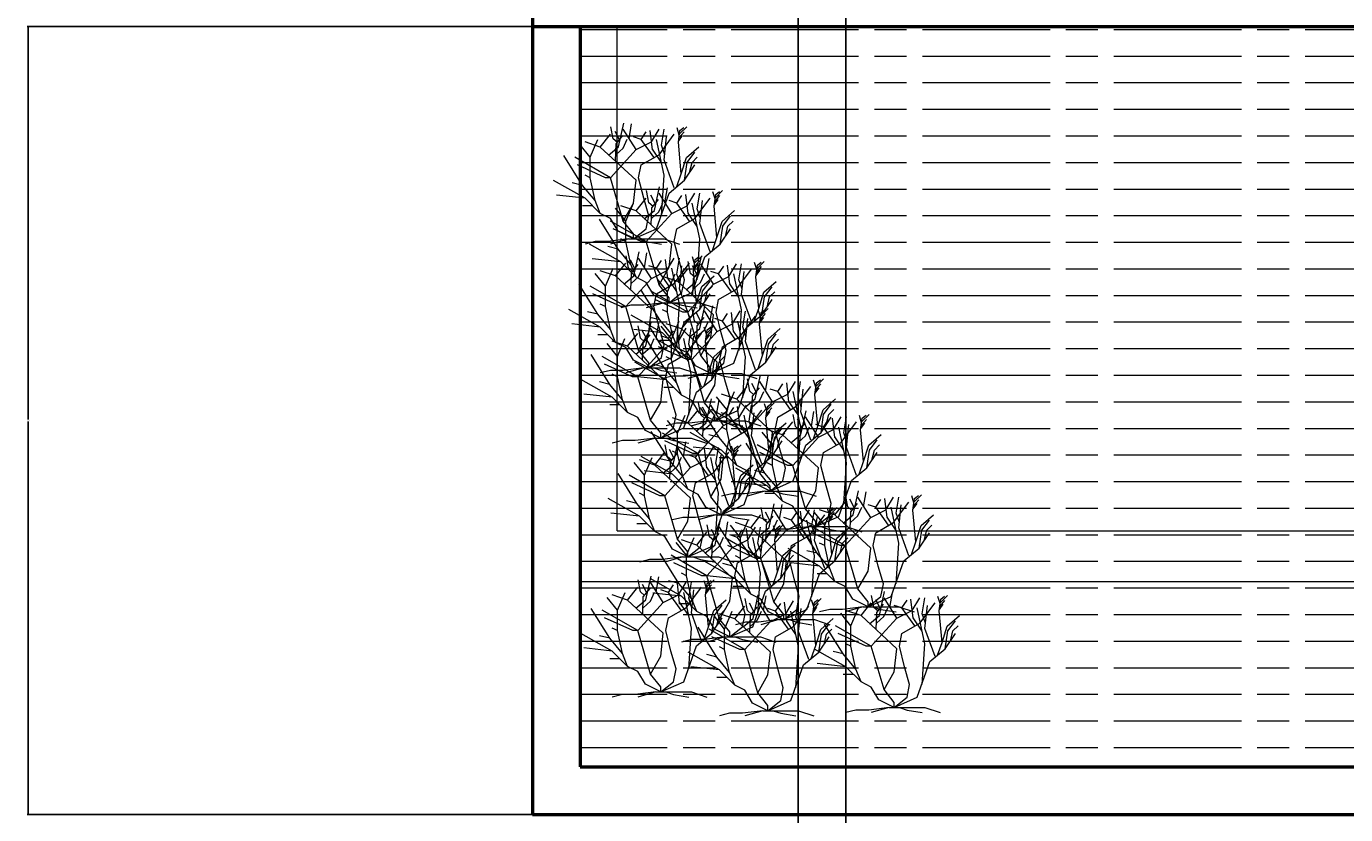
# Model space of a CAD drawing. Units: inches. Extents: x 5375 to 6084, y 16106 to 17259.
# Tile 2 of 32: x 5375 to 5624, y 16212 to 16361. Entities that reach past the tile are written whole.
import ezdxf

# ---------------------------------------------------------------- set-up
doc = ezdxf.new("R2010")
doc.units = ezdxf.units.IN
for name, color, linetype, lineweight in [('A-ANNO-DIMS', 2, 'Continuous', 18), ('C-PVMT-PATT', 2, 'Continuous', 13), ('L-PLNT-TREE', 3, 'Continuous', 13), ('WALL', 6, 'Continuous', 50)]:
    doc.layers.add(name, color=color, linetype=linetype, lineweight=lineweight)
doc.styles.get("Standard").update_dxf_attribs({"font": 'arial.ttf'})
doc.dimstyles.get("Standard").update_dxf_attribs({"dimtxt": 0.18, "dimasz": 0.18, "dimexe": 0.18, "dimexo": 0.0625, "dimgap": 0.09, "dimtad": 0, "dimtih": 1, "dimtoh": 1, "dimdec": 4, "dimzin": 0, "dimdsep": 46, "dimtxsty": 'Standard', "dimcen": 0.09, "dimadec": 0, "dimazin": 0, "dimtfac": 1, "dimtdec": 4, "dimtofl": 0, "dimtmove": 0, "dimatfit": 3, "dimfxl": 1, "dimtolj": 1, "dimtzin": 0, "dimarcsym": 0})

# ---------------------------------------------------------------- blocks, each defined once
blk = doc.blocks.new('*U12')
for p, q in [((-11.433, 18.289), (-10.457, 22.749)), ((-9.48, 19.775), (-8.992, 22.592)), ((-14.88, 18.24), (-12.96, 20.64)), ((-12.471, 19.775), (-12.898, 22.044)), ((-11.28, 19.619), (-12.104, 21.184)), ((-11.921, 18.836), (-10.64, 20.401)), ((-8.16, 17.76), (-10.56, 21.6)), ((-7.2, 19.68), (-8.64, 20.16)), ((-7.2, 19.68), (-6.24, 21.12)), ((-5.086, 17.741), (-5.513, 21.34)), ((-5.28, 19.2), (-3.84, 21.6)), ((-3.84, 16.8), (-0.96, 20.64)), ((-3.377, 18.602), (-2.888, 21.575)), ((-2.88, 15.84), (-2.4, 20.16)), ((-0.508, 21.888), (-0.081, 20.558)), ((-0.203, 19.149), (0.102, 21.34)), ((-0.142, 19.384), (0.59, 20.401)), ((-0.02, 20.01), (0.896, 21.105)), ((0.041, 20.714), (1.384, 22.044)), ((0.102, 21.34), (0.835, 21.888)), ((-16.8, 16.32), (-18.72, 18.72)), ((-14.88, 18.24), (-17.76, 19.2)), ((-16.8, 16.32), (-15.36, 19.68)), ((-8.16, 12), (-14.88, 18.24)), ((-13.325, 16.724), (-11.433, 18.289)), ((-12.96, 12.48), (-8.16, 17.76)), ((-11.677, 19.071), (-12.471, 19.775)), ((-12.043, 15.628), (-11.921, 18.836)), ((-11.982, 16.802), (-10.579, 18.054)), ((-10.579, 18.054), (-9.846, 19.697)), ((-8.16, 17.76), (-5.28, 19.2)), ((-4.8, 16.32), (-7.2, 19.68)), ((-3.377, 15.315), (-5.086, 17.819)), ((-2.88, 12.96), (-4.32, 19.68)), ((-2.766, 16.802), (-3.377, 18.602)), ((0.346, 13.203), (-0.203, 19.149)), ((1.323, 16.254), (3.642, 18.289)), ((-18.24, 11.04), (-21.755, 16.655)), ((-12.96, 12.48), (-19.68, 16.32)), ((-16.8, 12.48), (-16.8, 16.32)), ((-7.2, 14.88), (-3.84, 16.8)), ((-0.96, 10.56), (-2.88, 15.84)), ((0.346, 13.203), (1.323, 16.254)), ((0.96, 12), (1.44, 15.36)), ((1.44, 15.36), (2.88, 17.28)), ((1.92, 13.44), (2.4, 15.36)), ((2.4, 15.36), (3.36, 16.32)), ((-13.92, 12.48), (-19.2, 14.88)), ((-16.8, 12.48), (-17.76, 12.96)), ((-15.84, 8.16), (-16.8, 12.48)), ((-12.96, 12.48), (-13.92, 12.48)), ((-10.56, 4.32), (-12.96, 12.48)), ((-7.68, 12.48), (-7.2, 14.88)), ((-6.72, 8.64), (-7.68, 12.48)), ((-3.36, 5.28), (-2.88, 12.96)), ((-0.48, 10.8), (0.346, 13.203)), ((0.96, 12), (2.88, 14.88)), ((-17.76, 8.64), (-23.663, 11.961)), ((-18.24, 11.04), (-20.16, 11.52)), ((-15.84, 8.16), (-18.24, 11.04)), ((-8.64, 7.68), (-8.16, 12)), ((-1.92, 9.6), (0.96, 12)), ((-17.76, 8.64), (-23.128, 9.222)), ((-14.88, 5.76), (-17.76, 8.64)), ((-14.88, 5.76), (-15.84, 8.16)), ((-10.56, 4.32), (-8.64, 7.68)), ((-5.76, 5.28), (-6.72, 8.64)), ((-4.32, 2.88), (-1.92, 9.6)), ((-16.32, 7.2), (-18.24, 7.2)), ((-12.96, 4.8), (-14.88, 5.76)), ((-6.24, 2.88), (-5.76, 5.28)), ((-11.52, 2.4), (-12.96, 4.8)), ((-8.64, 1.92), (-10.56, 4.32)), ((-8.64, 0.96), (-4.32, 2.88)), ((-8.64, 0.96), (-6.24, 2.88)), ((-15.84, 0.48), (-17.76, 0)), ((-13.44, 0.48), (-15.84, 0.48)), ((-9.6, 0.96), (-13.44, 0.48)), ((-9.6, 0.96), (-12.96, 0)), ((-8.64, 0.96), (-11.52, 2.4)), ((-9.6, 0.96), (-7.68, 0.96)), ((-8.64, 0.96), (-8.64, 1.92)), ((-8.64, 0.96), (-2.88, 0.96)), ((-7.68, 0.96), (-6.24, 0.48)), ((-6.24, 0.48), (-3.36, 0)), ((-2.88, 0.96), (0, 0))]:
    blk.add_line(p, q)
blk = doc.blocks.new('*D33')
at = {"layer": 'A-ANNO-DIMS', "color": 0, "lineweight": -2, "transparency": 16777216}
for p, q in [((5470.56, 16360.58), (5375.56, 16360.58)), ((5375.74, 16360.4), (5375.74, 16286.66)), ((5375.74, 16212.56), (5375.74, 16286.3)), ((5470.56, 16212.38), (5375.56, 16212.38))]:
    blk.add_line(p, q, dxfattribs=at)
at = {"layer": 'A-ANNO-DIMS', "color": 0, "transparency": 16777216}
for points in [[(5375.71, 16360.4), (5375.77, 16360.4), (5375.74, 16360.58)], [(5375.71, 16212.56), (5375.77, 16212.56), (5375.74, 16212.38)]]:
    blk.add_solid(points, dxfattribs=at)
at = {"layer": 'Defpoints', "color": 0, "transparency": 16777216}
for p in [(5375.74, 16360.58), (5470.62, 16360.58), (5470.62, 16212.38)]:
    blk.add_point(p, dxfattribs=at)
at = {"layer": 'A-ANNO-DIMS', "color": 0, "transparency": 16777216, "insert": (5375.74, 16286.48), "char_height": 0.18, "attachment_point": 5}
blk.add_mtext('\\A1;148.2', dxfattribs=at)
blk = doc.blocks.new('*D40')
at = {"layer": 'A-ANNO-DIMS', "color": 0, "lineweight": -2, "transparency": 16777216}
for p, q in [((5529.62, 16876.52), (5529.62, 16106.48)), ((5520.62, 16867.52), (5520.62, 16106.48)), ((5520.8, 16106.66), (5524.97, 16106.66)), ((5529.44, 16106.66), (5525.27, 16106.66))]:
    blk.add_line(p, q, dxfattribs=at)
at = {"layer": 'A-ANNO-DIMS', "color": 0, "transparency": 16777216}
for points in [[(5520.8, 16106.69), (5520.8, 16106.63), (5520.62, 16106.66)], [(5529.44, 16106.69), (5529.44, 16106.63), (5529.62, 16106.66)]]:
    blk.add_solid(points, dxfattribs=at)
at = {"layer": 'Defpoints', "color": 0, "transparency": 16777216}
for p in [(5529.62, 16876.58), (5520.62, 16867.58), (5529.62, 16106.66)]:
    blk.add_point(p, dxfattribs=at)
at = {"layer": 'A-ANNO-DIMS', "color": 0, "transparency": 16777216, "insert": (5525.12, 16106.66), "char_height": 0.18, "attachment_point": 5}
blk.add_mtext('\\A1;9', dxfattribs=at)

msp = doc.modelspace()

# ---------------------------------------------------------------- hatches: boundary and pattern name
at = {"layer": 'C-PVMT-PATT'}
h = msp.add_hatch(dxfattribs=at)
h.set_pattern_fill('AR-B816C', color=256)
h.paths.add_polyline_path([(5707.6199, 16360.5793), (5479.6199, 16360.5793), (5479.6199, 16221.3785), (5802.2897, 16221.3785, 0.20288708), (5707.6199, 16299.0135)])
h = msp.add_hatch(dxfattribs=at)
h.set_pattern_fill('ACAD_ISO08W100', color=256)
h.paths.add_polyline_path([(5707.6199, 16360.5793), (5479.6199, 16360.5793), (5479.6199, 16221.3785), (5802.2897, 16221.3785, 0.20288708), (5707.6199, 16299.0135)])

# ---------------------------------------------------------------- linework, layer by layer
at = {"layer": 'WALL'}
for p, q in [((5470.6199, 16603.5793), (5470.6199, 16212.3785)), ((5470.6199, 16360.5793), (5707.6199, 16360.5793)), ((5479.6199, 16360.5793), (5479.6199, 16221.3785)), ((5479.6199, 16221.3785), (6022.6199, 16221.3785)), ((5470.6199, 16212.3785), (6031.6199, 16212.3785))]:
    msp.add_line(p, q, dxfattribs=at)

# ---------------------------------------------------------------- block references
at = {"layer": 'L-PLNT-TREE'}
for p in [(5498.2883, 16319.6538), (5505.0083, 16307.6538), (5501.1683, 16295.4138), (5512.8569, 16294.35), (5513.5769, 16285.47), (5503.4089, 16282.212), (5523.9837, 16272.2398), (5514.757, 16267.7776), (5532.5845, 16265.5668), (5508.517, 16259.8576), (5542.4264, 16250.4777), (5526.5864, 16248.0777), (5516.4184, 16244.8197), (5503.4193, 16234.4827), (5523.578, 16230.9501), (5547.3447, 16231.5511)]:
    msp.add_blockref('*U12', p, dxfattribs=at)

# ---------------------------------------------------------------- dimensions: what is measured, and where the dimension line sits
at = {"layer": 'A-ANNO-DIMS'}
dim = msp.add_linear_dim(base=(5529.6199, 16106.6631), p1=(5520.6199, 16867.5793), p2=(5529.6199, 16876.5793), dimstyle='Standard', override={"dimdec": 0, "dimlfac": 1, "dimrnd": 0, "dimzin": 0, "dimdsep": 46, "dimlunit": 2}, dxfattribs=at)
dim.commit()
dim.dimension.update_dxf_attribs({"geometry": '*D40', "text_midpoint": (5525.1199, 16106.6631)})
dim = msp.add_linear_dim(base=(5375.7423, 16360.5793), p1=(5470.6199, 16212.3785), p2=(5470.6199, 16360.5793), angle=90, dimstyle='Standard', override={"dimdec": 1, "dimlfac": 1, "dimrnd": 0, "dimzin": 0, "dimdsep": 46, "dimlunit": 2}, dxfattribs=at)
dim.commit()
dim.dimension.update_dxf_attribs({"geometry": '*D33', "text_midpoint": (5375.7423, 16286.4789)})

doc.saveas('drawing.dxf')
